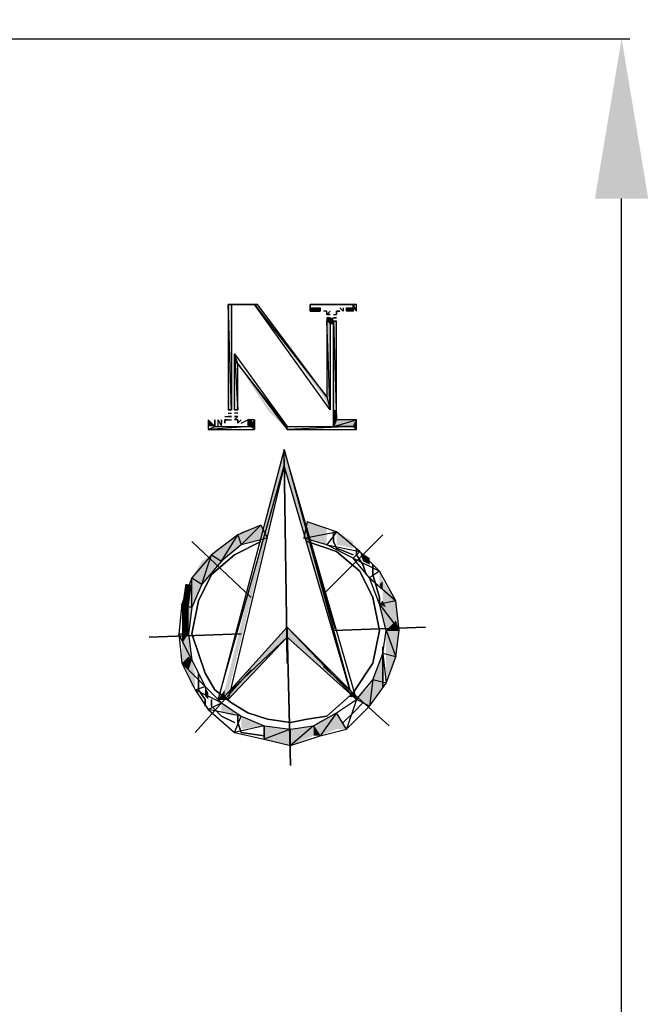
# Model space of a CAD drawing. Units: inches. Extents: x 1041 to 1781, y -140 to 732.
# Tile 5 of 6: x 1543 to 1638, y 358 to 506. Entities that reach past the tile are written whole.
import ezdxf

# ---------------------------------------------------------------- set-up
doc = ezdxf.new("R2010")
doc.units = ezdxf.units.IN
doc.layers.add('A-ANNO-SYMB', color=7, linetype='Continuous', lineweight=18)
doc.layers.add('dimension', color=130, linetype='Continuous', lineweight=18)
doc.layers.add('PDF_PDF3_PDF2_0', color=7, linetype='Continuous')
doc.styles.get("Standard").update_dxf_attribs({"font": 'arial.ttf'})
doc.dimstyles.new('ISO-25', dxfattribs={"dimtxt": 36, "dimasz": 24, "dimexe": 1.25, "dimexo": 0.625, "dimtad": 1, "dimlunit": 4, "dimtxsty": 'Standard', "dimcen": 2.5, "dimadec": 0, "dimazin": 0, "dimtfac": 1, "dimtmove": 0, "dimatfit": 3, "dimfxl": 1, "dimarcsym": 0})

# ---------------------------------------------------------------- blocks, each defined once
blk = doc.blocks.new('direction')
at = {"layer": 'PDF_PDF3_PDF2_0'}
for points in [[(4051.677, 1538.04), (4051.816, 1532.328), (4051.677, 1538.04)], [(4052.791, 1536.925), (4052.791, 1536.368), (4052.791, 1536.925)], [(4052.791, 1536.368), (4052.791, 1536.925), (4052.791, 1536.368)], [(4052.791, 1536.925), (4052.791, 1536.368), (4052.791, 1536.925)], [(4052.791, 1536.368), (4052.791, 1536.925), (4052.791, 1536.368)], [(4047.498, 1536.368), (4050.284, 1533.861), (4047.498, 1536.368)], [(4055.716, 1536.647), (4053.348, 1534), (4055.716, 1536.647)], [(4049.169, 1535.114), (4048.891, 1535.114), (4049.169, 1535.114)], [(4051.816, 1533.721), (4051.955, 1525.085), (4051.816, 1533.721)], [(4057.666, 1532.607), (4053.766, 1532.468), (4057.666, 1532.607)], [(4045.966, 1532.189), (4049.866, 1532.328), (4045.966, 1532.189)], [(4049.796, 1532.259), (4049.796, 1532.259), (4049.796, 1532.259), (4050.632, 1529.403)], [(4055.856, 1528.568), (4053.348, 1530.936), (4055.856, 1528.568)], [(4047.776, 1528.289), (4050.284, 1530.796), (4047.776, 1528.289)], [(4051.816, 1523.831), (4050.423, 1523.831), (4048.891, 1523.831)], [(4049.03, 1523.692), (4048.891, 1523.831), (4049.03, 1523.692)], [(4055.159, 1523.831), (4054.184, 1523.831), (4053.209, 1523.831), (4053.209, 1523.692), (4053.209, 1523.831)], [(4053.348, 1523.692), (4053.209, 1523.831), (4053.348, 1523.692)], [(4053.209, 1523.414), (4053.209, 1523.692), (4053.348, 1523.692), (4053.209, 1523.692)], [(4053.348, 1523.414), (4053.348, 1523.414), (4053.279, 1523.692)], [(4053.348, 1523.414), (4053.348, 1523.692), (4053.348, 1523.414)], [(4053.348, 1523.692), (4053.348, 1523.414), (4053.348, 1523.692)], [(4053.766, 1523.553), (4053.488, 1523.414), (4053.488, 1523.692)], [(4053.905, 1523.414), (4053.905, 1523.553), (4053.766, 1523.414)], [(4053.905, 1523.553), (4053.905, 1523.414), (4054.045, 1523.414), (4053.905, 1523.274), (4054.045, 1523.274), (4053.905, 1523.274), (4054.045, 1523.274)], [(4054.463, 1523.553), (4054.463, 1523.414), (4054.463, 1523.553), (4054.463, 1523.414), (4054.184, 1523.414)], [(4054.323, 1523.414), (4054.463, 1523.414), (4054.323, 1523.414)], [(4054.741, 1523.692), (4054.741, 1523.414), (4054.602, 1523.692), (4054.602, 1523.414), (4054.602, 1523.553)], [(4055.159, 1523.414), (4054.88, 1523.692), (4055.159, 1523.414), (4054.88, 1523.692)], [(4054.88, 1523.414), (4054.88, 1523.692), (4054.88, 1523.414)], [(4054.88, 1523.692), (4054.88, 1523.414), (4054.88, 1523.692)], [(4053.905, 1523.135), (4054.045, 1523.135)], [(4053.905, 1522.996), (4054.045, 1522.996), (4053.905, 1522.996)], [(4054.045, 1522.996), (4053.905, 1522.996), (4054.045, 1522.996)], [(4054.463, 1523.274), (4054.184, 1523.274), (4054.323, 1523.274), (4054.184, 1523.274)], [(4054.323, 1523.135), (4054.184, 1523.135)], [(4054.184, 1522.996), (4054.323, 1522.996), (4054.184, 1522.996)], [(4054.323, 1522.996), (4054.184, 1522.996), (4054.323, 1522.996)], [(4054.184, 1522.996), (4054.323, 1522.996), (4054.184, 1522.996)], [(4049.866, 1519.235), (4049.727, 1519.235)], [(4049.03, 1518.817), (4049.309, 1518.817), (4049.309, 1518.678), (4049.03, 1518.817), (4049.03, 1518.678), (4049.03, 1518.817), (4049.03, 1518.678), (4049.03, 1518.817), (4049.309, 1518.678), (4049.03, 1518.678), (4048.891, 1518.678), (4048.891, 1518.538)], [(4049.309, 1518.817), (4049.309, 1518.678), (4049.309, 1518.817), (4049.309, 1518.678)], [(4049.448, 1518.678), (4049.448, 1518.817), (4049.587, 1518.678)], [(4049.587, 1518.817), (4049.727, 1518.817), (4049.587, 1518.817)], [(4049.727, 1519.095), (4049.866, 1519.095), (4049.727, 1519.095)], [(4049.866, 1518.956), (4049.727, 1518.956), (4049.727, 1518.817), (4049.727, 1518.956)], [(4050.005, 1519.095), (4050.144, 1519.095), (4050.005, 1519.095), (4050.144, 1519.095), (4050.005, 1519.095), (4050.144, 1519.095)], [(4050.144, 1518.956), (4050.005, 1518.956), (4050.144, 1518.956)], [(4050.005, 1518.817), (4050.144, 1518.956), (4050.144, 1518.817), (4050.284, 1518.817)], [(4050.423, 1518.817), (4050.423, 1518.678), (4050.423, 1518.817)], [(4050.702, 1518.817), (4050.702, 1518.678), (4050.702, 1518.817)], [(4050.702, 1518.678), (4050.702, 1518.817), (4050.702, 1518.678)], [(4050.841, 1518.678), (4050.841, 1518.538), (4050.841, 1518.678)]]:
    blk.add_lwpolyline(points, dxfattribs=at)
for points in [[(4050.423, 1536.786), (4050.702, 1536.368), (4051.677, 1537.204)], [(4050.423, 1536.786), (4050.702, 1536.368), (4051.677, 1537.204)], [(4050.702, 1536.368), (4051.677, 1537.204), (4051.677, 1536.507)], [(4050.702, 1536.368), (4051.677, 1537.204), (4051.677, 1536.507)], [(4051.677, 1537.204), (4051.677, 1536.507), (4052.791, 1536.925)], [(4051.677, 1537.204), (4051.677, 1536.507), (4052.791, 1536.925)], [(4049.309, 1536.507), (4049.727, 1535.811), (4050.423, 1536.786)], [(4049.309, 1536.507), (4049.727, 1535.811), (4050.423, 1536.786)], [(4049.727, 1535.811), (4050.423, 1536.786), (4050.702, 1536.368)], [(4049.727, 1535.811), (4050.423, 1536.786), (4050.702, 1536.368)], [(4051.677, 1536.507), (4052.791, 1536.925), (4052.791, 1536.368)], [(4051.677, 1536.507), (4052.791, 1536.925), (4052.791, 1536.368)], [(4052.791, 1536.925), (4052.791, 1536.368), (4054.045, 1536.647)], [(4052.791, 1536.925), (4052.791, 1536.368), (4054.045, 1536.647)], [(4053.905, 1535.95), (4053.905, 1536.229), (4053.766, 1536.647), (4052.791, 1536.786), (4053.766, 1536.647), (4053.905, 1536.229)], [(4048.334, 1535.532), (4048.891, 1535.254), (4049.309, 1536.507)], [(4048.334, 1535.532), (4048.891, 1535.254), (4049.309, 1536.507)], [(4048.891, 1535.254), (4049.309, 1536.507), (4049.727, 1535.811)], [(4048.891, 1535.254), (4049.309, 1536.507), (4049.727, 1535.811)], [(4052.791, 1536.368), (4054.045, 1536.647), (4053.766, 1535.95)], [(4052.791, 1536.368), (4054.045, 1536.647), (4053.766, 1535.95)], [(4054.045, 1536.647), (4053.766, 1535.95), (4055.159, 1535.672)], [(4054.045, 1536.647), (4053.766, 1535.95), (4055.159, 1535.672)], [(4055.856, 1532.468), (4055.577, 1533.304), (4055.298, 1534.139), (4054.88, 1534.836), (4054.184, 1535.393), (4053.488, 1535.811), (4052.652, 1536.089), (4051.677, 1536.229), (4050.98, 1536.089), (4050.144, 1535.95), (4049.03, 1534.975), (4048.194, 1533.721), (4048.055, 1533.025), (4047.916, 1532.328), (4048.194, 1530.936), (4048.751, 1529.821), (4049.727, 1528.985), (4050.98, 1528.568), (4049.727, 1528.985), (4048.751, 1529.821), (4048.194, 1530.936), (4047.916, 1532.328), (4048.055, 1533.025), (4048.194, 1533.721), (4049.03, 1534.975), (4050.144, 1535.95), (4050.98, 1536.089), (4051.677, 1536.229), (4052.652, 1536.089), (4053.488, 1535.811), (4054.184, 1535.393), (4054.88, 1534.836), (4055.298, 1534.139), (4055.577, 1533.304), (4055.856, 1532.468), (4055.577, 1531.075), (4055.02, 1529.96), (4054.045, 1529.125), (4052.93, 1528.568), (4054.045, 1529.125), (4055.02, 1529.96), (4055.577, 1531.075)], [(4049.448, 1536.229), (4049.03, 1535.811), (4048.612, 1535.393), (4049.03, 1535.811)], [(4053.766, 1535.95), (4055.159, 1535.672), (4054.602, 1535.393)], [(4053.766, 1535.95), (4055.159, 1535.672), (4054.602, 1535.393)], [(4055.02, 1535.254), (4055.02, 1535.532), (4054.602, 1535.95), (4054.045, 1536.229), (4054.602, 1535.95), (4055.02, 1535.532)], [(4047.637, 1534.557), (4048.194, 1534.418), (4048.334, 1535.532)], [(4047.637, 1534.557), (4048.194, 1534.418), (4048.334, 1535.532)], [(4048.194, 1534.418), (4048.334, 1535.532), (4048.891, 1535.254)], [(4048.194, 1534.418), (4048.334, 1535.532), (4048.891, 1535.254)], [(4055.159, 1535.672), (4054.602, 1535.393), (4055.716, 1534.836)], [(4055.159, 1535.672), (4054.602, 1535.393), (4055.716, 1534.836)], [(4055.577, 1534.139), (4055.577, 1534.836), (4055.298, 1535.254), (4055.298, 1535.532), (4055.298, 1535.254), (4055.577, 1534.836)], [(4051.955, 1524.667), (4049.169, 1534.836), (4048.891, 1535.254)], [(4049.169, 1534.836), (4048.891, 1535.254), (4051.816, 1532.189)], [(4048.891, 1535.254), (4051.816, 1532.189), (4051.816, 1532.607)], [(4051.955, 1524.667), (4049.169, 1534.836), (4048.891, 1535.254)], [(4049.169, 1534.836), (4048.891, 1535.254), (4051.816, 1532.189)], [(4048.891, 1535.254), (4051.816, 1532.189), (4051.816, 1532.607)], [(4051.816, 1532.607), (4054.463, 1535.114), (4054.323, 1535.254)], [(4051.816, 1532.607), (4054.463, 1535.114), (4054.323, 1535.254)], [(4051.816, 1532.189), (4051.816, 1532.607), (4054.463, 1535.114)], [(4051.816, 1532.189), (4051.816, 1532.607), (4054.463, 1535.114)], [(4054.323, 1535.254), (4054.741, 1535.254), (4051.955, 1525.364)], [(4054.741, 1535.254), (4051.955, 1525.364), (4051.955, 1524.667)], [(4054.323, 1535.254), (4054.741, 1535.254), (4051.955, 1525.364)], [(4054.741, 1535.254), (4051.955, 1525.364), (4051.955, 1524.667)], [(4054.602, 1535.393), (4055.716, 1534.836), (4055.298, 1534.697)], [(4054.602, 1535.393), (4055.716, 1534.836), (4055.298, 1534.697)], [(4047.776, 1534.697), (4047.776, 1534), (4047.776, 1533.025), (4047.776, 1534)], [(4051.955, 1525.364), (4051.955, 1524.667), (4049.169, 1534.836)], [(4051.955, 1525.364), (4051.955, 1524.667), (4049.169, 1534.836)], [(4055.716, 1534.836), (4055.298, 1534.697), (4056.273, 1533.721)], [(4055.716, 1534.836), (4055.298, 1534.697), (4056.273, 1533.721)], [(4055.298, 1534.697), (4056.273, 1533.721), (4055.856, 1533.582)], [(4055.298, 1534.697), (4056.273, 1533.721), (4055.856, 1533.582)], [(4047.219, 1533.443), (4047.776, 1533.304), (4047.637, 1534.557)], [(4047.219, 1533.443), (4047.776, 1533.304), (4047.637, 1534.557)], [(4047.776, 1533.304), (4047.637, 1534.557), (4048.194, 1534.418)], [(4047.776, 1533.304), (4047.637, 1534.557), (4048.194, 1534.418)], [(4047.08, 1532.328), (4047.637, 1532.328), (4047.219, 1533.443)], [(4047.08, 1532.328), (4047.637, 1532.328), (4047.219, 1533.443)], [(4047.637, 1532.328), (4047.219, 1533.443), (4047.776, 1533.304)], [(4047.637, 1532.328), (4047.219, 1533.443), (4047.776, 1533.304)], [(4056.273, 1533.721), (4055.856, 1533.582), (4056.413, 1532.468)], [(4056.273, 1533.721), (4055.856, 1533.582), (4056.413, 1532.468)], [(4055.856, 1533.582), (4056.413, 1532.468), (4055.995, 1532.468)], [(4055.856, 1533.582), (4056.413, 1532.468), (4055.995, 1532.468)], [(4047.219, 1531.075), (4047.916, 1531.214), (4047.08, 1532.328)], [(4047.916, 1531.214), (4047.08, 1532.328), (4047.637, 1532.328)], [(4047.219, 1531.075), (4047.916, 1531.214), (4047.08, 1532.328)], [(4047.916, 1531.214), (4047.08, 1532.328), (4047.637, 1532.328)], [(4055.995, 1532.468), (4056.273, 1531.214), (4055.856, 1531.353)], [(4055.995, 1532.468), (4056.273, 1531.214), (4055.856, 1531.353)], [(4056.413, 1532.468), (4055.995, 1532.468), (4056.273, 1531.214)], [(4056.413, 1532.468), (4055.995, 1532.468), (4056.273, 1531.214)], [(4055.856, 1531.353), (4055.856, 1530.1), (4055.438, 1530.378)], [(4055.856, 1531.353), (4055.856, 1530.1), (4055.438, 1530.378)], [(4056.273, 1531.214), (4055.856, 1531.353), (4055.856, 1530.1)], [(4056.273, 1531.214), (4055.856, 1531.353), (4055.856, 1530.1)], [(4048.334, 1530.1), (4047.219, 1531.075), (4047.916, 1531.214)], [(4048.334, 1530.1), (4047.219, 1531.075), (4047.916, 1531.214)], [(4047.916, 1529.821), (4048.334, 1530.1), (4047.219, 1531.075)], [(4047.916, 1529.821), (4048.334, 1530.1), (4047.219, 1531.075)], [(4048.194, 1529.543), (4048.194, 1529.96), (4047.916, 1530.936), (4047.916, 1531.214), (4047.916, 1530.936), (4048.194, 1529.96)], [(4049.03, 1529.264), (4047.916, 1529.821), (4048.334, 1530.1)], [(4049.03, 1529.264), (4047.916, 1529.821), (4048.334, 1530.1)], [(4055.438, 1530.378), (4055.02, 1529.125), (4054.602, 1529.403)], [(4055.438, 1530.378), (4055.02, 1529.125), (4054.602, 1529.403)], [(4055.856, 1530.1), (4055.438, 1530.378), (4055.02, 1529.125)], [(4055.856, 1530.1), (4055.438, 1530.378), (4055.02, 1529.125)], [(4048.751, 1528.985), (4049.03, 1529.264), (4047.916, 1529.821)], [(4048.751, 1528.985), (4049.03, 1529.264), (4047.916, 1529.821)], [(4048.891, 1528.846), (4048.891, 1529.125), (4048.612, 1529.543), (4048.473, 1529.96), (4048.612, 1529.543), (4048.891, 1529.125)], [(4050.144, 1528.707), (4048.751, 1528.985), (4049.03, 1529.264)], [(4050.144, 1528.707), (4048.751, 1528.985), (4049.03, 1529.264)], [(4054.602, 1529.403), (4053.905, 1528.289), (4053.766, 1528.707)], [(4054.602, 1529.403), (4053.905, 1528.289), (4053.766, 1528.707)], [(4055.02, 1529.125), (4054.602, 1529.403), (4053.905, 1528.289)], [(4055.02, 1529.125), (4054.602, 1529.403), (4053.905, 1528.289)], [(4049.727, 1528.15), (4050.144, 1528.707), (4048.751, 1528.985)], [(4049.727, 1528.15), (4050.144, 1528.707), (4048.751, 1528.985)], [(4049.866, 1528.15), (4049.866, 1528.568), (4049.727, 1528.846), (4049.03, 1529.125), (4049.727, 1528.846), (4049.866, 1528.568)], [(4051.119, 1528.428), (4049.727, 1528.15), (4050.144, 1528.707)], [(4051.119, 1528.428), (4049.727, 1528.15), (4050.144, 1528.707)], [(4050.98, 1527.732), (4051.119, 1528.428), (4049.727, 1528.15)], [(4050.98, 1527.732), (4051.119, 1528.428), (4049.727, 1528.15)], [(4053.766, 1528.707), (4052.93, 1527.871), (4052.652, 1528.428)], [(4053.766, 1528.707), (4052.93, 1527.871), (4052.652, 1528.428)], [(4053.905, 1528.289), (4053.766, 1528.707), (4052.93, 1527.871)], [(4053.905, 1528.289), (4053.766, 1528.707), (4052.93, 1527.871)], [(4048.891, 1523.414), (4049.03, 1523.692), (4048.891, 1523.831)], [(4048.891, 1523.831), (4049.03, 1523.692), (4051.816, 1523.831)], [(4049.03, 1523.692), (4051.816, 1523.831), (4051.816, 1523.692)], [(4051.816, 1523.831), (4051.816, 1523.692), (4053.905, 1521.046)], [(4053.209, 1523.414), (4053.348, 1523.692), (4053.209, 1523.831)], [(4053.209, 1523.831), (4053.348, 1523.692), (4055.159, 1523.831)], [(4053.348, 1523.692), (4055.159, 1523.831), (4054.88, 1523.692)], [(4055.159, 1523.831), (4054.88, 1523.692), (4055.159, 1523.414)], [(4049.727, 1523.414), (4049.866, 1523.692), (4048.891, 1523.414)], [(4049.866, 1523.692), (4048.891, 1523.414), (4049.03, 1523.692)], [(4049.866, 1519.235), (4049.727, 1523.414), (4049.866, 1523.692)], [(4049.727, 1519.235), (4049.866, 1519.235), (4049.727, 1523.414)], [(4051.816, 1523.692), (4053.905, 1521.046), (4054.045, 1520.628)], [(4053.348, 1523.414), (4053.348, 1523.692), (4053.209, 1523.414)], [(4053.348, 1523.692), (4053.209, 1523.414), (4053.209, 1523.692)], [(4053.488, 1523.414), (4053.488, 1523.692), (4053.348, 1523.414)], [(4053.488, 1523.692), (4053.348, 1523.414), (4053.348, 1523.692)], [(4053.209, 1518.538), (4050.144, 1522.438), (4050.005, 1522.996)], [(4050.144, 1522.438), (4050.005, 1522.996), (4050.144, 1519.235)], [(4050.005, 1522.996), (4050.144, 1519.235), (4050.005, 1519.235)], [(4053.905, 1521.046), (4054.045, 1520.628), (4053.905, 1522.996)], [(4054.045, 1520.628), (4053.905, 1522.996), (4054.045, 1522.996)], [(4054.323, 1522.996), (4054.184, 1522.996), (4054.323, 1518.538)], [(4054.184, 1522.996), (4054.323, 1518.538), (4054.184, 1518.538)], [(4053.07, 1518.538), (4053.209, 1518.538), (4050.144, 1522.438)], [(4050.144, 1519.235), (4050.005, 1519.235), (4050.144, 1519.095)], [(4050.005, 1519.235), (4050.144, 1519.095), (4050.005, 1519.095)], [(4048.891, 1518.538), (4049.03, 1518.538), (4048.891, 1518.817)], [(4049.03, 1518.538), (4048.891, 1518.817), (4049.03, 1518.678)], [(4050.423, 1518.817), (4050.423, 1518.678), (4050.702, 1518.817)], [(4050.423, 1518.678), (4050.702, 1518.817), (4050.702, 1518.678)], [(4050.702, 1518.817), (4050.702, 1518.678), (4050.841, 1518.817)], [(4050.702, 1518.678), (4050.841, 1518.817), (4050.841, 1518.678)], [(4050.841, 1518.817), (4050.841, 1518.678), (4050.841, 1518.538)], [(4050.841, 1518.538), (4049.03, 1518.538), (4048.891, 1518.538), (4050.841, 1518.538), (4048.891, 1518.538)], [(4054.323, 1518.538), (4054.184, 1518.538), (4053.07, 1518.538)], [(4054.184, 1518.538), (4053.07, 1518.538), (4053.209, 1518.538)]]:
    blk.add_lwpolyline(points, close=True, dxfattribs=at)
at = {"layer": 'PDF_PDF3_PDF2_0', "const_width": 0.276}
blk.add_lwpolyline([(4055.995, 1530.378), (4056.134, 1531.353), (4056.134, 1532.468)], dxfattribs=at)
at = {"layer": 'PDF_PDF3_PDF2_0', "transparency": 33554559}
for points in [[(4050.702, 1536.786), (4050.702, 1536.368), (4051.677, 1537.204)], [(4050.702, 1536.368), (4051.677, 1537.204), (4051.677, 1536.507)], [(4050.702, 1536.786), (4050.702, 1536.368), (4051.677, 1537.204)], [(4050.702, 1536.368), (4051.677, 1537.204), (4051.677, 1536.507)], [(4051.677, 1537.204), (4051.677, 1536.507), (4052.791, 1536.925)], [(4051.677, 1537.204), (4051.677, 1536.507), (4052.791, 1536.925)], [(4049.727, 1536.507), (4049.727, 1535.811), (4050.423, 1536.786)], [(4049.727, 1535.811), (4050.423, 1536.786), (4050.562, 1536.229)], [(4049.727, 1536.507), (4049.727, 1535.811), (4050.423, 1536.786)], [(4049.727, 1535.811), (4050.423, 1536.786), (4050.562, 1536.229)], [(4050.423, 1536.786), (4050.562, 1536.229), (4050.702, 1536.368)], [(4050.423, 1536.786), (4050.702, 1536.786), (4050.702, 1536.368)], [(4050.423, 1536.786), (4050.562, 1536.229), (4050.702, 1536.368)], [(4050.423, 1536.786), (4050.702, 1536.786), (4050.702, 1536.368)], [(4051.677, 1536.507), (4052.791, 1536.925), (4052.791, 1536.368)], [(4051.677, 1536.507), (4052.791, 1536.925), (4052.791, 1536.925)], [(4051.677, 1536.507), (4052.791, 1536.925), (4052.791, 1536.368)], [(4051.677, 1536.507), (4052.791, 1536.925), (4052.791, 1536.925)], [(4049.309, 1536.507), (4049.727, 1536.507), (4049.727, 1535.811)], [(4049.309, 1536.507), (4049.727, 1536.507), (4049.727, 1535.811)], [(4052.791, 1536.368), (4053.766, 1536.507), (4053.766, 1535.95)], [(4052.791, 1536.368), (4053.766, 1536.507), (4053.766, 1535.95)], [(4054.045, 1535.95), (4054.045, 1535.811), (4054.602, 1535.811)], [(4054.045, 1535.95), (4054.045, 1535.811), (4054.602, 1535.811)], [(4048.194, 1535.254), (4048.194, 1534.418), (4048.334, 1535.532)], [(4048.194, 1534.418), (4048.334, 1535.532), (4048.334, 1534.697)], [(4048.194, 1535.254), (4048.194, 1534.418), (4048.334, 1535.532)], [(4048.194, 1534.418), (4048.334, 1535.532), (4048.334, 1534.697)], [(4048.334, 1535.532), (4048.334, 1534.697), (4048.891, 1535.254)], [(4048.334, 1535.532), (4048.334, 1534.697), (4048.891, 1535.254)], [(4054.045, 1535.811), (4054.602, 1535.811), (4054.602, 1535.393)], [(4054.045, 1535.811), (4054.602, 1535.811), (4054.602, 1535.393)], [(4047.776, 1534.697), (4047.776, 1534.557), (4048.194, 1535.254)], [(4047.776, 1534.557), (4048.194, 1535.254), (4048.194, 1534.418)], [(4047.776, 1534.697), (4047.776, 1534.557), (4048.194, 1535.254)], [(4047.776, 1534.557), (4048.194, 1535.254), (4048.194, 1534.418)], [(4051.816, 1532.607), (4054.323, 1535.254), (4054.323, 1534.975)], [(4051.816, 1532.607), (4054.323, 1535.254), (4054.323, 1534.975)], [(4054.323, 1534.975), (4054.323, 1535.254), (4054.323, 1535.114)], [(4054.323, 1535.254), (4054.463, 1535.254), (4054.463, 1535.254)], [(4054.323, 1535.254), (4054.323, 1535.114), (4054.323, 1535.114)], [(4054.323, 1535.114), (4054.323, 1535.114), (4054.323, 1535.254)], [(4054.323, 1534.975), (4054.323, 1535.254), (4054.323, 1535.114)], [(4054.323, 1535.254), (4054.463, 1535.254), (4054.463, 1535.254)], [(4054.323, 1535.254), (4054.323, 1535.114), (4054.323, 1535.114)], [(4054.323, 1535.114), (4054.323, 1535.114), (4054.323, 1535.254)], [(4054.323, 1534.975), (4054.323, 1535.114), (4054.323, 1535.114)], [(4054.323, 1535.114), (4054.463, 1535.114), (4054.463, 1535.114)], [(4054.323, 1534.975), (4054.323, 1534.418), (4054.463, 1535.114)], [(4054.323, 1534.418), (4054.463, 1535.114), (4054.463, 1534.836)], [(4054.323, 1534.975), (4054.323, 1535.114), (4054.323, 1535.114)], [(4054.323, 1535.114), (4054.463, 1535.114), (4054.463, 1535.114)], [(4054.323, 1534.975), (4054.323, 1534.418), (4054.463, 1535.114)], [(4054.323, 1534.418), (4054.463, 1535.114), (4054.463, 1534.836)], [(4054.463, 1535.254), (4054.463, 1535.114), (4054.463, 1535.114)], [(4054.741, 1535.254), (4054.741, 1535.254), (4054.463, 1534.836)], [(4054.741, 1535.254), (4054.463, 1534.836), (4054.463, 1535.254)], [(4054.463, 1535.254), (4054.463, 1535.114), (4054.463, 1535.114)], [(4054.741, 1535.254), (4054.741, 1535.254), (4054.463, 1534.836)], [(4054.741, 1535.254), (4054.463, 1534.836), (4054.463, 1535.254)], [(4054.463, 1535.114), (4054.463, 1534.836), (4054.463, 1534.836)], [(4054.463, 1534.836), (4054.463, 1534.836), (4054.463, 1535.114)], [(4054.463, 1535.114), (4054.463, 1534.836), (4054.463, 1534.836)], [(4054.463, 1534.836), (4054.463, 1534.836), (4054.463, 1535.114)], [(4055.159, 1535.254), (4055.159, 1534.975), (4055.298, 1535.114)], [(4055.159, 1535.254), (4055.159, 1534.975), (4055.298, 1535.114)], [(4055.159, 1534.975), (4055.298, 1535.114), (4055.298, 1534.697)], [(4055.159, 1534.975), (4055.298, 1535.114), (4055.298, 1534.697)], [(4049.169, 1534.836), (4049.169, 1534.975), (4051.816, 1532.189)], [(4049.169, 1534.975), (4051.816, 1532.607), (4051.816, 1532.189)], [(4049.169, 1534.836), (4049.169, 1534.975), (4051.816, 1532.189)], [(4049.169, 1534.975), (4051.816, 1532.607), (4051.816, 1532.189)], [(4049.169, 1534.836), (4051.955, 1525.364), (4051.955, 1524.667)], [(4049.169, 1534.836), (4051.955, 1525.364), (4051.955, 1524.667)], [(4054.323, 1534.975), (4054.323, 1534.975), (4051.816, 1532.189)], [(4054.323, 1534.975), (4051.816, 1532.189), (4051.816, 1532.607)], [(4054.323, 1534.975), (4054.323, 1534.975), (4051.816, 1532.189)], [(4054.323, 1534.975), (4051.816, 1532.189), (4051.816, 1532.607)], [(4051.955, 1525.364), (4054.323, 1534.975), (4054.323, 1534.418)], [(4051.955, 1525.364), (4054.323, 1534.975), (4054.323, 1534.418)], [(4054.323, 1534.975), (4054.323, 1534.418), (4054.323, 1534.418)], [(4054.323, 1534.418), (4054.323, 1534.418), (4054.323, 1534.975)], [(4054.323, 1534.975), (4054.323, 1534.418), (4054.323, 1534.418)], [(4054.323, 1534.418), (4054.323, 1534.418), (4054.323, 1534.975)], [(4054.463, 1534.836), (4054.463, 1534.836), (4054.323, 1534.279)], [(4054.463, 1534.836), (4054.323, 1534.279), (4054.323, 1534.418)], [(4054.463, 1534.836), (4054.463, 1534.836), (4054.323, 1534.279)], [(4054.463, 1534.836), (4054.323, 1534.279), (4054.323, 1534.418)], [(4055.716, 1534.836), (4055.716, 1534.139), (4055.856, 1534.697)], [(4055.716, 1534.836), (4055.716, 1534.139), (4055.856, 1534.697)], [(4055.716, 1534.139), (4055.856, 1534.697), (4055.995, 1534)], [(4055.716, 1534.139), (4055.856, 1534.697), (4055.995, 1534)], [(4055.995, 1534), (4056.273, 1533.721), (4055.856, 1534.697)], [(4055.995, 1534), (4056.273, 1533.721), (4055.856, 1534.697)], [(4047.637, 1534.418), (4047.219, 1533.443), (4047.637, 1533.304)], [(4047.637, 1534.418), (4047.219, 1533.443), (4047.637, 1533.304)], [(4047.637, 1534.557), (4047.637, 1534.557), (4047.637, 1533.304)], [(4047.637, 1534.557), (4047.637, 1533.304), (4047.637, 1534.418)], [(4047.637, 1534.557), (4047.637, 1534.557), (4047.637, 1533.304)], [(4047.637, 1534.557), (4047.637, 1533.304), (4047.637, 1534.418)], [(4047.776, 1533.304), (4047.776, 1534.557), (4048.194, 1534.418)], [(4047.776, 1533.304), (4047.776, 1534.557), (4048.194, 1534.418)], [(4051.955, 1525.364), (4051.955, 1524.667), (4054.323, 1534.418)], [(4051.955, 1524.667), (4054.323, 1534.418), (4054.323, 1534.279)], [(4051.955, 1525.364), (4051.955, 1524.667), (4054.323, 1534.418)], [(4051.955, 1524.667), (4054.323, 1534.418), (4054.323, 1534.279)], [(4055.716, 1534.139), (4055.856, 1533.582), (4055.995, 1534)], [(4055.716, 1534.139), (4055.856, 1533.582), (4055.995, 1534)], [(4055.856, 1533.582), (4055.995, 1534), (4055.995, 1533.582)], [(4055.856, 1533.582), (4055.995, 1534), (4055.995, 1533.582)], [(4055.995, 1533.582), (4055.995, 1534), (4056.273, 1533.721)], [(4055.995, 1533.582), (4055.995, 1534), (4056.273, 1533.721)], [(4047.08, 1532.328), (4047.219, 1533.443), (4047.219, 1532.328)], [(4047.08, 1532.328), (4047.219, 1533.443), (4047.219, 1532.328)], [(4047.219, 1533.443), (4047.219, 1532.328), (4047.637, 1532.328)], [(4047.219, 1533.443), (4047.637, 1533.304), (4047.637, 1532.328)], [(4047.219, 1533.443), (4047.219, 1532.328), (4047.637, 1532.328)], [(4047.219, 1533.443), (4047.637, 1533.304), (4047.637, 1532.328)], [(4055.995, 1533.582), (4055.856, 1533.582), (4055.995, 1533.443)], [(4055.856, 1533.582), (4055.995, 1533.443), (4055.995, 1532.468)], [(4055.995, 1533.582), (4055.856, 1533.582), (4055.995, 1533.443)], [(4055.856, 1533.582), (4055.995, 1533.443), (4055.995, 1532.468)], [(4055.995, 1533.582), (4055.995, 1533.443), (4056.273, 1533.721)], [(4055.995, 1533.443), (4056.273, 1533.721), (4056.273, 1532.886)], [(4055.995, 1533.582), (4055.995, 1533.443), (4056.273, 1533.721)], [(4055.995, 1533.443), (4056.273, 1533.721), (4056.273, 1532.886)], [(4055.995, 1533.443), (4055.995, 1532.468), (4056.273, 1532.886)], [(4055.995, 1533.443), (4055.995, 1532.468), (4056.273, 1532.886)], [(4047.637, 1532.328), (4047.637, 1533.304), (4047.637, 1532.746)], [(4047.637, 1532.328), (4047.637, 1533.304), (4047.637, 1532.746)], [(4055.995, 1532.468), (4056.273, 1532.886), (4056.273, 1532.468)], [(4055.995, 1532.468), (4056.273, 1532.886), (4056.273, 1532.468)], [(4047.219, 1532.328), (4047.08, 1532.328), (4047.219, 1531.911)], [(4047.08, 1532.328), (4047.219, 1531.911), (4047.219, 1531.075)], [(4047.219, 1532.328), (4047.08, 1532.328), (4047.219, 1531.911)], [(4047.08, 1532.328), (4047.219, 1531.911), (4047.219, 1531.075)], [(4047.219, 1532.328), (4047.219, 1531.911), (4047.637, 1532.328)], [(4047.219, 1531.911), (4047.637, 1532.328), (4047.637, 1531.353)], [(4047.219, 1532.328), (4047.219, 1531.911), (4047.637, 1532.328)], [(4047.219, 1531.911), (4047.637, 1532.328), (4047.637, 1531.353)], [(4047.637, 1531.353), (4047.916, 1531.214), (4047.637, 1532.328)], [(4047.637, 1531.353), (4047.916, 1531.214), (4047.637, 1532.328)], [(4055.856, 1531.353), (4055.995, 1532.468), (4055.995, 1531.214)], [(4055.995, 1532.468), (4055.995, 1531.214), (4055.856, 1531.353)], [(4056.273, 1532.468), (4055.995, 1532.468), (4056.273, 1531.214)], [(4055.995, 1532.468), (4056.273, 1531.214), (4055.995, 1531.493)], [(4047.219, 1531.911), (4047.219, 1531.075), (4047.637, 1531.353)], [(4047.219, 1531.911), (4047.219, 1531.075), (4047.637, 1531.353)], [(4047.219, 1531.075), (4047.637, 1531.353), (4047.776, 1531.075)], [(4047.219, 1531.075), (4047.637, 1531.353), (4047.776, 1531.075)], [(4047.776, 1531.075), (4047.637, 1531.353), (4047.916, 1531.214)], [(4047.776, 1531.075), (4047.637, 1531.353), (4047.916, 1531.214)], [(4055.438, 1530.378), (4055.856, 1531.353), (4055.856, 1530.1)], [(4055.438, 1530.378), (4055.856, 1531.353), (4055.856, 1530.1)], [(4055.995, 1531.493), (4056.134, 1530.378), (4055.856, 1530.378)], [(4055.856, 1530.1), (4055.856, 1531.353), (4055.995, 1531.214)], [(4055.995, 1531.214), (4055.856, 1531.353), (4055.856, 1530.1)], [(4056.273, 1531.214), (4055.995, 1531.493), (4056.134, 1530.378)], [(4047.776, 1531.075), (4047.219, 1531.075), (4047.776, 1530.657)], [(4047.219, 1531.075), (4047.776, 1530.657), (4047.776, 1530.239)], [(4047.776, 1531.075), (4047.219, 1531.075), (4047.776, 1530.657)], [(4047.219, 1531.075), (4047.776, 1530.657), (4047.776, 1530.239)], [(4047.776, 1530.657), (4047.776, 1530.239), (4047.916, 1530.378)], [(4047.776, 1530.657), (4047.776, 1530.239), (4047.916, 1530.378)], [(4047.776, 1530.239), (4047.916, 1530.378), (4047.916, 1529.821)], [(4047.776, 1530.239), (4047.916, 1530.378), (4047.916, 1529.821)], [(4055.02, 1529.821), (4055.02, 1529.125), (4055.438, 1530.378)], [(4055.02, 1529.125), (4055.438, 1530.378), (4055.438, 1529.403)], [(4055.02, 1529.821), (4055.02, 1529.125), (4055.438, 1530.378)], [(4055.02, 1529.125), (4055.438, 1530.378), (4055.438, 1529.403)], [(4055.438, 1530.378), (4055.438, 1529.403), (4055.856, 1530.1)], [(4055.438, 1530.378), (4055.438, 1529.403), (4055.856, 1530.1)], [(4054.602, 1529.403), (4055.02, 1529.821), (4055.02, 1529.125)], [(4054.602, 1529.403), (4055.02, 1529.821), (4055.02, 1529.125)], [(4048.334, 1529.543), (4048.334, 1529.264), (4048.612, 1529.403)], [(4048.334, 1529.543), (4048.334, 1529.264), (4048.612, 1529.403)], [(4048.334, 1529.264), (4048.612, 1529.403), (4048.751, 1528.985)], [(4048.334, 1529.264), (4048.612, 1529.403), (4048.751, 1528.985)], [(4053.905, 1528.846), (4053.905, 1528.289), (4054.602, 1529.403)], [(4053.905, 1528.289), (4054.602, 1529.403), (4054.741, 1528.846)], [(4053.905, 1528.846), (4053.905, 1528.289), (4054.602, 1529.403)], [(4053.905, 1528.289), (4054.602, 1529.403), (4054.741, 1528.846)], [(4054.602, 1529.403), (4054.741, 1528.846), (4055.02, 1529.125)], [(4054.602, 1529.403), (4054.741, 1528.846), (4055.02, 1529.125)], [(4049.03, 1528.846), (4049.03, 1528.568), (4049.727, 1528.707)], [(4049.03, 1528.846), (4049.03, 1528.568), (4049.727, 1528.707)], [(4053.766, 1528.707), (4053.905, 1528.846), (4053.905, 1528.289)], [(4053.766, 1528.707), (4053.905, 1528.846), (4053.905, 1528.289)], [(4049.03, 1528.568), (4049.727, 1528.707), (4049.727, 1528.15)], [(4049.03, 1528.568), (4049.727, 1528.707), (4049.727, 1528.15)], [(4050.98, 1528.428), (4050.144, 1528.15), (4050.144, 1528.707)], [(4050.98, 1528.428), (4050.144, 1528.15), (4050.144, 1528.707)], [(4050.98, 1528.428), (4050.98, 1528.428), (4050.144, 1528.15)], [(4050.144, 1528.15), (4050.144, 1528.01), (4050.98, 1528.428)], [(4050.144, 1528.01), (4050.98, 1528.428), (4050.98, 1527.732)], [(4050.98, 1528.428), (4050.98, 1528.428), (4050.144, 1528.15)], [(4050.144, 1528.15), (4050.144, 1528.01), (4050.98, 1528.428)], [(4050.144, 1528.01), (4050.98, 1528.428), (4050.98, 1527.732)], [(4050.98, 1527.732), (4050.98, 1528.428), (4051.119, 1528.428)], [(4050.98, 1528.428), (4051.119, 1528.428), (4051.119, 1528.428)], [(4050.98, 1527.732), (4050.98, 1528.428), (4051.119, 1528.428)], [(4050.98, 1528.428), (4051.119, 1528.428), (4051.119, 1528.428)], [(4052.652, 1528.428), (4052.791, 1528.428), (4052.93, 1527.871)], [(4052.652, 1528.428), (4052.791, 1528.428), (4052.93, 1527.871)], [(4052.791, 1528.428), (4052.93, 1527.871), (4053.766, 1528.707)], [(4052.791, 1528.428), (4052.93, 1527.871), (4053.766, 1528.707)], [(4052.93, 1527.871), (4053.766, 1528.707), (4053.766, 1528.15)], [(4052.93, 1527.871), (4053.766, 1528.707), (4053.766, 1528.15)], [(4053.766, 1528.707), (4053.766, 1528.15), (4053.905, 1528.289)], [(4053.766, 1528.707), (4053.766, 1528.15), (4053.905, 1528.289)], [(4048.891, 1523.692), (4049.03, 1523.692), (4048.891, 1523.831)], [(4049.727, 1523.414), (4049.866, 1523.692), (4048.891, 1523.414)], [(4049.866, 1523.692), (4048.891, 1523.414), (4049.03, 1523.692)], [(4048.891, 1523.414), (4049.03, 1523.692), (4048.891, 1523.692)], [(4048.891, 1523.692), (4048.891, 1523.692), (4049.03, 1523.692)], [(4049.866, 1523.414), (4049.727, 1523.414), (4049.866, 1523.692)], [(4049.727, 1522.996), (4049.727, 1523.414), (4049.727, 1523.414)], [(4049.866, 1522.996), (4049.866, 1523.414), (4049.727, 1523.414)], [(4049.866, 1522.996), (4049.727, 1522.996), (4049.727, 1523.414)], [(4051.816, 1523.692), (4052.512, 1522.996), (4052.512, 1522.996)], [(4052.512, 1522.996), (4052.512, 1522.996), (4051.816, 1523.692)], [(4052.512, 1522.996), (4052.652, 1522.996), (4051.816, 1523.692)], [(4052.652, 1522.996), (4051.816, 1523.692), (4051.955, 1523.692)], [(4053.209, 1523.414), (4053.209, 1523.692), (4053.348, 1523.692)], [(4053.209, 1523.692), (4053.348, 1523.692), (4053.348, 1523.692)], [(4053.348, 1523.692), (4053.348, 1523.692), (4053.209, 1523.692)], [(4053.488, 1523.414), (4053.348, 1523.414), (4053.488, 1523.692)], [(4053.348, 1523.414), (4053.488, 1523.692), (4053.348, 1523.692)], [(4055.159, 1523.414), (4054.88, 1523.692), (4055.159, 1523.692)], [(4054.88, 1523.692), (4055.159, 1523.692), (4055.159, 1523.692)], [(4055.159, 1523.692), (4055.159, 1523.692), (4054.88, 1523.692)], [(4054.88, 1523.692), (4054.88, 1523.414), (4054.88, 1523.414)], [(4054.88, 1523.414), (4054.88, 1523.414), (4054.88, 1523.692)], [(4049.727, 1522.996), (4049.727, 1522.996), (4049.866, 1520.628)], [(4049.727, 1522.996), (4049.866, 1520.628), (4049.727, 1520.628)], [(4049.866, 1520.628), (4049.727, 1522.996), (4049.866, 1522.996)], [(4050.284, 1522.438), (4050.144, 1522.438), (4050.005, 1522.996)], [(4050.144, 1522.438), (4050.005, 1522.996), (4050.005, 1522.438)], [(4053.905, 1521.046), (4052.512, 1522.996), (4052.652, 1522.996)], [(4052.512, 1522.996), (4053.905, 1521.046), (4053.905, 1521.046)], [(4053.905, 1521.046), (4053.905, 1521.046), (4052.512, 1522.996)], [(4054.045, 1521.046), (4053.905, 1521.046), (4053.905, 1522.996)], [(4053.905, 1522.996), (4054.045, 1522.996), (4054.045, 1522.996)], [(4054.045, 1522.996), (4054.045, 1522.996), (4053.905, 1522.996)], [(4054.045, 1521.046), (4053.905, 1522.996), (4054.045, 1522.996)], [(4054.323, 1522.438), (4054.184, 1522.438), (4054.184, 1522.996)], [(4054.323, 1518.538), (4054.184, 1522.996), (4054.323, 1522.996)], [(4050.144, 1519.235), (4050.005, 1522.438), (4050.144, 1522.438)], [(4050.005, 1522.438), (4050.005, 1522.438), (4050.144, 1519.235)], [(4050.005, 1522.438), (4050.144, 1519.235), (4050.005, 1519.235)], [(4052.652, 1519.235), (4052.512, 1519.235), (4050.144, 1522.438)], [(4052.652, 1519.235), (4050.144, 1522.438), (4050.284, 1522.438)], [(4054.184, 1518.538), (4054.323, 1518.538), (4054.184, 1522.438)], [(4054.323, 1518.538), (4054.184, 1522.438), (4054.323, 1522.438)], [(4054.045, 1521.046), (4054.045, 1520.628), (4053.905, 1521.046)], [(4054.045, 1520.628), (4053.905, 1521.046), (4053.905, 1521.046)], [(4054.045, 1521.046), (4054.045, 1521.046), (4054.045, 1520.628)], [(4049.727, 1519.235), (4049.866, 1519.235), (4049.727, 1520.628)], [(4049.866, 1519.235), (4049.727, 1520.628), (4049.866, 1520.628)], [(4049.866, 1519.235), (4049.866, 1520.628), (4049.866, 1520.628)], [(4049.866, 1519.235), (4050.144, 1519.235), (4049.866, 1519.374)], [(4050.144, 1519.235), (4049.866, 1519.374), (4050.005, 1519.374)], [(4049.866, 1519.095), (4050.005, 1519.095), (4049.866, 1519.235)], [(4050.005, 1519.095), (4049.866, 1519.235), (4050.144, 1519.235)], [(4050.144, 1519.095), (4050.005, 1519.095), (4050.005, 1519.235)], [(4050.144, 1519.095), (4050.005, 1519.235), (4050.144, 1519.235)], [(4053.07, 1518.538), (4053.209, 1518.538), (4052.512, 1519.235)], [(4053.209, 1518.538), (4052.512, 1519.235), (4052.652, 1519.235)], [(4053.209, 1518.538), (4052.652, 1519.235), (4052.652, 1519.235)], [(4049.309, 1518.817), (4049.309, 1518.678), (4049.03, 1518.817)], [(4049.309, 1518.678), (4049.03, 1518.817), (4049.03, 1518.678)], [(4049.309, 1518.817), (4049.309, 1518.817), (4049.309, 1518.678)], [(4050.005, 1519.095), (4050.144, 1519.095), (4050.144, 1519.095)], [(4050.144, 1519.095), (4050.144, 1519.095), (4050.005, 1519.095)], [(4050.702, 1518.678), (4050.423, 1518.678), (4050.702, 1518.817)], [(4050.423, 1518.678), (4050.702, 1518.817), (4050.423, 1518.817)], [(4050.702, 1518.817), (4050.423, 1518.817), (4050.423, 1518.817)], [(4050.841, 1518.817), (4050.841, 1518.678), (4050.702, 1518.678)], [(4050.702, 1518.817), (4050.702, 1518.817), (4050.702, 1518.678)], [(4050.702, 1518.817), (4050.702, 1518.678), (4050.841, 1518.817)], [(4050.841, 1518.817), (4050.841, 1518.817), (4050.841, 1518.678)], [(4048.891, 1518.538), (4048.891, 1518.538), (4050.841, 1518.538)], [(4048.891, 1518.538), (4050.841, 1518.538), (4049.03, 1518.538)], [(4048.891, 1518.538), (4049.03, 1518.538), (4049.03, 1518.538)], [(4049.03, 1518.538), (4049.03, 1518.678), (4049.03, 1518.678)], [(4050.841, 1518.538), (4050.841, 1518.678), (4050.841, 1518.678)], [(4050.841, 1518.678), (4050.841, 1518.538), (4050.841, 1518.538)], [(4050.841, 1518.538), (4050.841, 1518.538), (4050.841, 1518.678)], [(4054.184, 1518.538), (4054.323, 1518.538), (4053.07, 1518.538)], [(4054.184, 1518.538), (4053.07, 1518.538), (4053.209, 1518.538)], [(4054.184, 1518.538), (4054.184, 1518.538), (4054.323, 1518.538)]]:
    blk.add_solid(points, dxfattribs=at)
blk = doc.blocks.new('*D16')
at = {"layer": 'Defpoints', "color": 0, "transparency": 16777216}
for p in [(1498.75, 503.23), (1633.79, 503.23), (1498.75, 32.23)]:
    blk.add_point(p, dxfattribs=at)
at = {"layer": 'dimension', "color": 0, "lineweight": -2, "transparency": 16777216}
for p, q in [((1499.37, 503.23), (1635.04, 503.23)), ((1633.79, 56.23), (1633.79, 479.23)), ((1499.37, 32.23), (1635.04, 32.23))]:
    blk.add_line(p, q, dxfattribs=at)
at = {"layer": 'dimension', "color": 0, "transparency": 16777216}
for points in [[(1629.79, 479.23), (1637.79, 479.23), (1633.79, 503.23)], [(1629.79, 56.23), (1637.79, 56.23), (1633.79, 32.23)]]:
    blk.add_solid(points, dxfattribs=at)
at = {"layer": 'dimension', "color": 0, "transparency": 16777216, "insert": (1614.78, 267.73), "char_height": 36, "attachment_point": 5, "rotation": 90}
blk.add_mtext('39\'-3"', dxfattribs=at)
blk = doc.blocks.new('*D18')
at = {"layer": 'Defpoints', "color": 0, "transparency": 16777216}
for p in [(1449.44, 541.68), (1413.44, 207.73), (1449.44, 207.73)]:
    blk.add_point(p, dxfattribs=at)
at = {"layer": 'dimension', "color": 0, "lineweight": -2, "transparency": 16777216}
for p, q in [((1413.44, 208.36), (1413.44, 542.93)), ((1449.44, 208.36), (1449.44, 542.93)), ((1389.44, 541.68), (1365.44, 541.68)), ((1413.44, 541.68), (1449.44, 541.68)), ((1473.44, 541.68), (1594.36, 541.68))]:
    blk.add_line(p, q, dxfattribs=at)
at = {"layer": 'dimension', "color": 0, "transparency": 16777216}
for points in [[(1389.44, 545.68), (1389.44, 537.68), (1413.44, 541.68)], [(1473.44, 545.68), (1473.44, 537.68), (1449.44, 541.68)]]:
    blk.add_solid(points, dxfattribs=at)
at = {"layer": 'dimension', "color": 0, "transparency": 16777216, "insert": (1545.9, 560.7), "char_height": 36, "attachment_point": 5}
blk.add_mtext('3\'-0"', dxfattribs=at)
blk = doc.blocks.new('*D20')
at = {"layer": 'Defpoints', "color": 0, "transparency": 16777216}
for p in [(1425.44, 395.23), (1449.44, 395.23), (1449.44, 2.78)]:
    blk.add_point(p, dxfattribs=at)
at = {"layer": 'dimension', "color": 0, "lineweight": -2, "transparency": 16777216}
for p, q in [((1425.44, 394.61), (1425.44, 1.53)), ((1449.44, 394.61), (1449.44, 1.53)), ((1401.44, 2.78), (1377.44, 2.78)), ((1425.44, 2.78), (1449.44, 2.78)), ((1473.44, 2.78), (1595, 2.78))]:
    blk.add_line(p, q, dxfattribs=at)
at = {"layer": 'dimension', "color": 0, "transparency": 16777216}
for points in [[(1401.44, 6.78), (1401.44, -1.22), (1425.44, 2.78)], [(1473.44, 6.78), (1473.44, -1.22), (1449.44, 2.78)]]:
    blk.add_solid(points, dxfattribs=at)
at = {"layer": 'dimension', "color": 0, "transparency": 16777216, "insert": (1546.22, 21.79), "char_height": 36, "attachment_point": 5}
blk.add_mtext('2\'-0"', dxfattribs=at)
blk = doc.blocks.new('*D21')
at = {"layer": 'Defpoints', "color": 0, "transparency": 16777216}
for p in [(1449.44, 541.68), (1410.44, 41.23), (1449.44, 41.23)]:
    blk.add_point(p, dxfattribs=at)
at = {"layer": 'dimension', "color": 0, "lineweight": -2, "transparency": 16777216}
for p, q in [((1410.44, 41.86), (1410.44, 542.93)), ((1449.44, 41.86), (1449.44, 542.93)), ((1386.44, 541.68), (1362.44, 541.68)), ((1410.44, 541.68), (1449.44, 541.68)), ((1473.44, 541.68), (1594.36, 541.68))]:
    blk.add_line(p, q, dxfattribs=at)
at = {"layer": 'dimension', "color": 0, "transparency": 16777216}
for points in [[(1386.44, 545.68), (1386.44, 537.68), (1410.44, 541.68)], [(1473.44, 545.68), (1473.44, 537.68), (1449.44, 541.68)]]:
    blk.add_solid(points, dxfattribs=at)
at = {"layer": 'dimension', "color": 0, "transparency": 16777216, "insert": (1545.9, 560.7), "char_height": 36, "attachment_point": 5}
blk.add_mtext('3\'-3"', dxfattribs=at)
blk = doc.blocks.new('*D31')
at = {"layer": 'Defpoints', "color": 0, "transparency": 16777216}
for p in [(1390.94, 447.73), (1427, 447.73), (1427, 2.78)]:
    blk.add_point(p, dxfattribs=at)
at = {"layer": 'dimension', "color": 0, "lineweight": -2, "transparency": 16777216}
for p, q in [((1390.94, 447.11), (1390.94, 1.53)), ((1427, 447.11), (1427, 1.53)), ((1366.94, 2.78), (1342.94, 2.78)), ((1390.94, 2.78), (1427, 2.78)), ((1451, 2.78), (1571.93, 2.78))]:
    blk.add_line(p, q, dxfattribs=at)
at = {"layer": 'dimension', "color": 0, "transparency": 16777216}
for points in [[(1366.94, 6.78), (1366.94, -1.22), (1390.94, 2.78)], [(1451, 6.78), (1451, -1.22), (1427, 2.78)]]:
    blk.add_solid(points, dxfattribs=at)
at = {"layer": 'dimension', "color": 0, "transparency": 16777216, "insert": (1523.46, 21.8), "char_height": 36, "attachment_point": 5}
blk.add_mtext('3\'-0"', dxfattribs=at)
blk = doc.blocks.new('*D39')
at = {"layer": 'Defpoints', "color": 0, "transparency": 16777216}
for p in [(1467.44, 541.68), (1449.44, 207.73), (1467.44, 207.73)]:
    blk.add_point(p, dxfattribs=at)
at = {"layer": 'dimension', "color": 0, "lineweight": -2, "transparency": 16777216}
for p, q in [((1449.44, 208.36), (1449.44, 542.93)), ((1467.44, 208.36), (1467.44, 542.93)), ((1425.44, 541.68), (1401.44, 541.68)), ((1449.44, 541.68), (1467.44, 541.68)), ((1491.44, 541.68), (1609, 541.68))]:
    blk.add_line(p, q, dxfattribs=at)
at = {"layer": 'dimension', "color": 0, "transparency": 16777216}
for points in [[(1425.44, 545.68), (1425.44, 537.68), (1449.44, 541.68)], [(1491.44, 545.68), (1491.44, 537.68), (1467.44, 541.68)]]:
    blk.add_solid(points, dxfattribs=at)
at = {"layer": 'dimension', "color": 0, "transparency": 16777216, "insert": (1562.22, 560.69), "char_height": 36, "attachment_point": 5}
blk.add_mtext('1\'-6"', dxfattribs=at)

msp = doc.modelspace()

# ---------------------------------------------------------------- block references
at = {"layer": 'A-ANNO-SYMB', "xscale": 3.548028847586577, "yscale": 3.548028847586577, "zscale": 3.548028847586577, "rotation": 180}
msp.add_blockref('direction', (15959.547, 5851.148), dxfattribs=at)

# ---------------------------------------------------------------- dimensions: what is measured, and where the dimension line sits
at = {"layer": 'dimension'}
for base, p1, p2, picture, middle in [((1449.438, 541.683), (1410.438, 41.233), (1449.438, 41.233), '*D21', (1545.899, 560.7)), ((1449.438, 541.683), (1413.438, 207.733), (1449.438, 207.733), '*D18', (1545.899, 560.7)), ((1467.438, 541.683), (1449.438, 207.733), (1467.438, 207.733), '*D39', (1562.217, 560.688)), ((1427.003, 2.783), (1390.938, 447.733), (1427.003, 447.733), '*D31', (1523.464, 21.8)), ((1449.438, 2.783), (1425.438, 395.233), (1449.438, 395.233), '*D20', (1546.218, 21.788))]:
    dim = msp.add_linear_dim(base=base, p1=p1, p2=p2, dimstyle='ISO-25', override={"dimdec": 1, "dimlfac": 1, "dimrnd": 0, "dimzin": 1, "dimdsep": 46, "dimlunit": 4, "dimfrac": 2}, dxfattribs=at)
    dim.commit()
    dim.dimension.update_dxf_attribs({"geometry": picture, "text_midpoint": middle})
dim = msp.add_linear_dim(base=(1633.794, 503.233), p1=(1498.749, 32.233), p2=(1498.749, 503.233), angle=90, dimstyle='ISO-25', override={"dimdec": 1, "dimlfac": 1, "dimrnd": 0, "dimzin": 1, "dimdsep": 46, "dimlunit": 4, "dimfrac": 2}, dxfattribs=at)
dim.commit()
dim.dimension.update_dxf_attribs({"geometry": '*D16', "text_midpoint": (1614.777, 267.733)})

doc.saveas('drawing.dxf')
